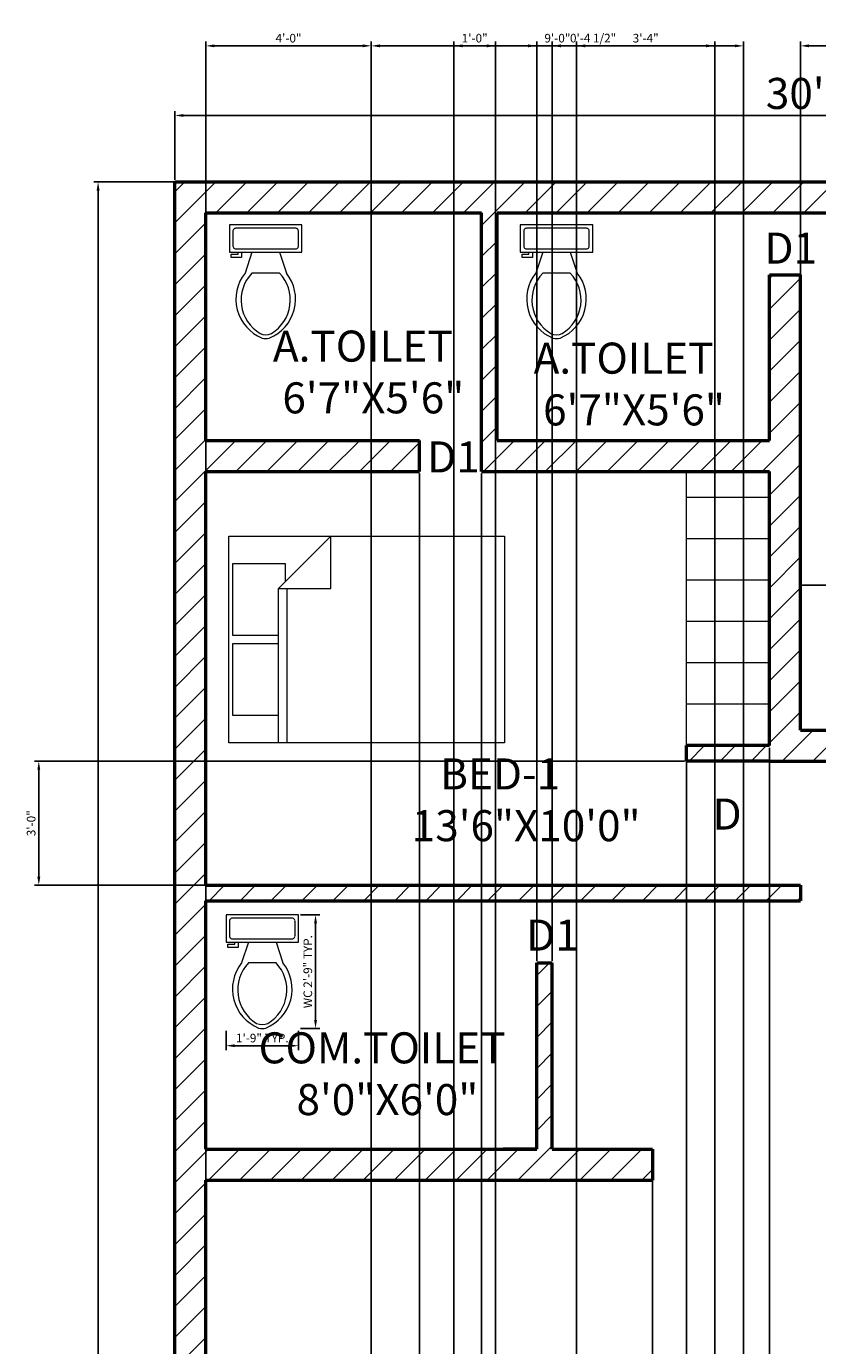
# Model space of a CAD drawing. Units: inches. Extents: x 2758 to 3288, y 1211 to 2050.
# Tile 3 of 4: x 2758 to 2988, y 1667 to 2050. Entities that reach past the tile are written whole.
import ezdxf

# ---------------------------------------------------------------- set-up
doc = ezdxf.new("R2010")
doc.units = ezdxf.units.IN
for name, color, linetype, lineweight in [('A-ANNO-DIMS', 2, 'Continuous', 18), ('A-AREA-IDEN', 7, 'Continuous', 25), ('A-FLOR-FIXT', 9, 'Continuous', 18), ('A-FURN', 8, 'Continuous', 18), ('A-WALL', 7, 'Continuous', 50)]:
    doc.layers.add(name, color=color, linetype=linetype, lineweight=lineweight)
for name, color, linetype, lineweight, true_color in [('A-ANNO-TEXT', 244, 'Continuous', 18, 0x991b1e), ('A-FLOR-CASE', 244, 'Continuous', 18, 0x991b1e), ('A-WALL-PATT', 244, 'Continuous', 13, 0x991b1e)]:
    doc.layers.add(name, color=color, linetype=linetype, lineweight=lineweight, true_color=true_color)
doc.styles.get("Standard").update_dxf_attribs({"font": 'arial.ttf'})
doc.dimstyles.new('ISO-25', dxfattribs={"dimtxt": 2.5, "dimasz": 2.5, "dimexe": 1.25, "dimexo": 0.625, "dimtad": 1, "dimlunit": 3, "dimtxsty": 'Standard', "dimcen": 2.5, "dimadec": 0, "dimazin": 0, "dimtfac": 1, "dimtmove": 0, "dimatfit": 3, "dimfxl": 1, "dimarcsym": 0})

# ---------------------------------------------------------------- blocks, each defined once
blk = doc.blocks.new('Bed - Queen')
for p, q in [((0, -80.00003), (0, 0)), ((0, 0), (59.99999, 0)), ((59.99999, 0), (59.99999, -80.00003)), ((7.99999, -1.2), (28.79998, -1.2)), ((7.99999, -14.4), (7.99999, -1.2)), ((28.79998, -1.2), (28.79998, -14.4)), ((31.19999, -1.2), (51.99999, -1.2)), ((31.19999, -14.4), (31.19999, -1.2)), ((51.99999, -1.2), (51.99999, -16.4)), ((0, -14.4), (44.8, -14.4)), ((59.99999, -29.6), (44.8, -14.4)), ((44.8, -14.4), (44.8, -29.6)), ((44.8, -16.8), (0, -16.8)), ((51.99999, -16.4), (46.79936, -16.4)), ((44.8, -29.6), (59.99999, -29.6)), ((59.99999, -80.00003), (0, -80.00003))]:
    blk.add_line(p, q)
blk = doc.blocks.new('Toilet - top')
for p, q in [((9.5, -6), (9.5, -2)), ((-10, -8.5), (-8, -8.5)), ((-10, -9.5), (-10, -8.5)), ((-7, -9.5), (-10, -9.5)), ((-8, -8.5), (-8, -8)), ((-7, -8), (-7, -9.5)), ((-4, -8), (-6, -14)), ((4, -8), (6, -14)), ((4, -14), (-4, -14))]:
    blk.add_line(p, q)
blk.add_lwpolyline([(10.5, -8), (10.5, 0), (-10.5, 0), (-10.5, -8)], close=True)
for points in [[(-9.5, -2), (-9.5, -6)], [(8.5, -1), (-8.5, -1)], [(-8.5, -7), (8.5, -7)]]:
    blk.add_lwpolyline(points)
for centre, radius, start, end in [((-8.62, -1.88), 0.884, 81.8699, 188.1301), ((8.62, -1.88), 0.884, 351.8699, 98.1301), ((-8.62, -6.12), 0.884, 171.8699, 278.1301), ((8.62, -6.12), 0.884, 261.8699, 8.1301), ((3.52, -21.58), 12.17, 141.4691, 247.9714), ((4.2, -21.82), 11.33, 136.3677, 238.9468), ((-3.52, -21.58), 12.17, 292.0284, 38.5307), ((-4.2, -21.82), 11.33, 301.053, 43.6321), ((0, -27.88), 4, 245.7318, 294.2682), ((0, -29), 4, 254.8605, 285.1395)]:
    blk.add_arc(centre, radius, start, end)
blk = doc.blocks.new('*D6')
at = {"layer": 'A-ANNO-DIMS', "color": 0, "lineweight": -2, "transparency": 16777216}
for p, q in [((2801.14, 2005.44), (2801.14, 2025.32)), ((2803.64, 2024.07), (3158.64, 2024.07)), ((3161.14, 2005.44), (3161.14, 2025.32))]:
    blk.add_line(p, q, dxfattribs=at)
at = {"layer": 'A-ANNO-DIMS', "color": 0, "transparency": 16777216}
for points in [[(2803.64, 2024.49), (2803.64, 2023.65), (2801.14, 2024.07)], [(3158.64, 2024.49), (3158.64, 2023.65), (3161.14, 2024.07)]]:
    blk.add_solid(points, dxfattribs=at)
at = {"layer": 'Defpoints', "color": 0, "transparency": 16777216}
for p in [(3161.14, 2024.07), (2801.14, 2004.81), (3161.14, 2004.81)]:
    blk.add_point(p, dxfattribs=at)
at = {"layer": 'A-ANNO-DIMS', "color": 0, "transparency": 16777216, "insert": (2981.14, 2029.29), "char_height": 9, "attachment_point": 5}
blk.add_mtext("30'", dxfattribs=at)
blk = doc.blocks.new('*D7')
at = {"layer": 'A-ANNO-DIMS', "color": 0, "lineweight": -2, "transparency": 16777216}
for p, q in [((2801.18, 2004.81), (2777.63, 2004.81)), ((2778.88, 2002.31), (2778.88, 1287.31)), ((2800.51, 1284.81), (2777.63, 1284.81))]:
    blk.add_line(p, q, dxfattribs=at)
at = {"layer": 'A-ANNO-DIMS', "color": 0, "transparency": 16777216}
for points in [[(2778.47, 2002.31), (2779.3, 2002.31), (2778.88, 2004.81)], [(2778.47, 1287.31), (2779.3, 1287.31), (2778.88, 1284.81)]]:
    blk.add_solid(points, dxfattribs=at)
at = {"layer": 'Defpoints', "color": 0, "transparency": 16777216}
for p in [(2801.81, 2004.81), (2778.88, 1284.81), (2801.14, 1284.81)]:
    blk.add_point(p, dxfattribs=at)
at = {"layer": 'A-ANNO-DIMS', "color": 0, "transparency": 16777216, "insert": (2773.66, 1644.81), "char_height": 9, "attachment_point": 5, "rotation": 90}
blk.add_mtext("60'", dxfattribs=at)
blk = doc.blocks.new('*D10')
at = {"layer": 'A-ANNO-DIMS', "color": 0, "lineweight": -2, "transparency": 16777216}
for p, q in [((2837.64, 1792.28), (2843.22, 1792.28)), ((2841.97, 1761.74), (2841.97, 1789.78)), ((2837.64, 1759.24), (2843.22, 1759.24))]:
    blk.add_line(p, q, dxfattribs=at)
at = {"layer": 'A-ANNO-DIMS', "color": 0, "transparency": 16777216}
for points in [[(2841.56, 1789.78), (2842.39, 1789.78), (2841.97, 1792.28)], [(2841.56, 1761.74), (2842.39, 1761.74), (2841.97, 1759.24)]]:
    blk.add_solid(points, dxfattribs=at)
at = {"layer": 'Defpoints', "color": 0, "transparency": 16777216}
for p in [(2837.02, 1792.28), (2841.97, 1792.28), (2837.02, 1759.24)]:
    blk.add_point(p, dxfattribs=at)
at = {"layer": 'A-ANNO-DIMS', "color": 0, "transparency": 16777216, "insert": (2840.06, 1775.76), "char_height": 2.5, "attachment_point": 5, "rotation": 90}
blk.add_mtext('WC 2\'-9" TYP.', dxfattribs=at)
blk = doc.blocks.new('*D11')
at = {"layer": 'A-ANNO-DIMS', "color": 0, "lineweight": -2, "transparency": 16777216}
for p, q in [((2816.02, 1758.61), (2816.02, 1753.03)), ((2837.02, 1758.61), (2837.02, 1753.03)), ((2818.52, 1754.28), (2834.52, 1754.28))]:
    blk.add_line(p, q, dxfattribs=at)
at = {"layer": 'A-ANNO-DIMS', "color": 0, "transparency": 16777216}
for points in [[(2818.52, 1754.7), (2818.52, 1753.86), (2816.02, 1754.28)], [(2834.52, 1754.7), (2834.52, 1753.86), (2837.02, 1754.28)]]:
    blk.add_solid(points, dxfattribs=at)
at = {"layer": 'Defpoints', "color": 0, "transparency": 16777216}
for p in [(2816.02, 1759.24), (2837.02, 1759.24), (2837.02, 1754.28)]:
    blk.add_point(p, dxfattribs=at)
at = {"layer": 'A-ANNO-DIMS', "color": 0, "transparency": 16777216, "insert": (2826.52, 1756.18), "char_height": 2.5, "attachment_point": 5}
blk.add_mtext('1\'-9" TYP.', dxfattribs=at)
blk = doc.blocks.new('*D23')
at = {"layer": 'A-ANNO-DIMS', "color": 0, "lineweight": -2, "transparency": 16777216}
for p, q in [((2903.64, 2044.26), (2901.14, 2044.26)), ((2906.14, 1778.94), (2906.14, 2045.51)), ((2906.14, 2044.26), (2910.64, 2044.26)), ((2910.64, 1778.94), (2910.64, 2045.51)), ((2913.14, 2044.26), (2929.36, 2044.26))]:
    blk.add_line(p, q, dxfattribs=at)
at = {"layer": 'A-ANNO-DIMS', "color": 0, "transparency": 16777216}
for points in [[(2903.64, 2044.68), (2903.64, 2043.84), (2906.14, 2044.26)], [(2913.14, 2044.68), (2913.14, 2043.84), (2910.64, 2044.26)]]:
    blk.add_solid(points, dxfattribs=at)
at = {"layer": 'Defpoints', "color": 0, "transparency": 16777216}
for p in [(2910.64, 2044.26), (2906.14, 1778.31), (2910.64, 1778.31)]:
    blk.add_point(p, dxfattribs=at)
at = {"layer": 'A-ANNO-DIMS', "color": 0, "transparency": 16777216, "insert": (2922.5, 2046.18), "char_height": 2.5, "attachment_point": 5}
blk.add_mtext('0\'-4 1/2"', dxfattribs=at)
blk = doc.blocks.new('*D24')
at = {"layer": 'A-ANNO-DIMS', "color": 0, "lineweight": -2, "transparency": 16777216}
for p, q in [((2872.14, 1920.19), (2872.14, 1211.4)), ((2890.14, 1920.19), (2890.14, 1211.4)), ((2874.64, 1212.65), (2887.64, 1212.65))]:
    blk.add_line(p, q, dxfattribs=at)
at = {"layer": 'A-ANNO-DIMS', "color": 0, "transparency": 16777216}
for points in [[(2874.64, 1213.06), (2874.64, 1212.23), (2872.14, 1212.65)], [(2887.64, 1213.06), (2887.64, 1212.23), (2890.14, 1212.65)]]:
    blk.add_solid(points, dxfattribs=at)
at = {"layer": 'Defpoints', "color": 0, "transparency": 16777216}
for p in [(2872.14, 1920.81), (2890.14, 1920.81), (2890.14, 1212.65)]:
    blk.add_point(p, dxfattribs=at)
at = {"layer": 'A-ANNO-DIMS', "color": 0, "transparency": 16777216, "insert": (2881.14, 1214.55), "char_height": 2.5, "attachment_point": 5}
blk.add_mtext('1\'-6"', dxfattribs=at)
blk = doc.blocks.new('*D26')
at = {"layer": 'A-ANNO-DIMS', "color": 0, "lineweight": -2, "transparency": 16777216}
for p, q in [((2949.01, 1836.81), (2760.44, 1836.81)), ((2761.69, 1803.31), (2761.69, 1834.31)), ((2982.01, 1800.81), (2760.44, 1800.81))]:
    blk.add_line(p, q, dxfattribs=at)
at = {"layer": 'A-ANNO-DIMS', "color": 0, "transparency": 16777216}
for points in [[(2761.27, 1834.31), (2762.11, 1834.31), (2761.69, 1836.81)], [(2761.27, 1803.31), (2762.11, 1803.31), (2761.69, 1800.81)]]:
    blk.add_solid(points, dxfattribs=at)
at = {"layer": 'Defpoints', "color": 0, "transparency": 16777216}
for p in [(2761.69, 1836.81), (2949.64, 1836.81), (2982.64, 1800.81)]:
    blk.add_point(p, dxfattribs=at)
at = {"layer": 'A-ANNO-DIMS', "color": 0, "transparency": 16777216, "insert": (2759.79, 1818.81), "char_height": 2.5, "attachment_point": 5, "rotation": 90}
blk.add_mtext('3\'-0"', dxfattribs=at)
blk = doc.blocks.new('*D28')
at = {"layer": 'A-ANNO-DIMS', "color": 0, "lineweight": -2, "transparency": 16777216}
for p, q in [((2939.69, 1723.69), (2939.69, 1211.4)), ((3011.14, 1723.69), (3011.14, 1211.4)), ((2942.19, 1212.65), (3008.64, 1212.65))]:
    blk.add_line(p, q, dxfattribs=at)
at = {"layer": 'A-ANNO-DIMS', "color": 0, "transparency": 16777216}
for points in [[(2942.19, 1213.06), (2942.19, 1212.23), (2939.69, 1212.65)], [(3008.64, 1213.06), (3008.64, 1212.23), (3011.14, 1212.65)]]:
    blk.add_solid(points, dxfattribs=at)
at = {"layer": 'Defpoints', "color": 0, "transparency": 16777216}
for p in [(2939.69, 1724.31), (3011.14, 1724.31), (3011.14, 1212.65)]:
    blk.add_point(p, dxfattribs=at)
at = {"layer": 'A-ANNO-DIMS', "color": 0, "transparency": 16777216, "insert": (2975.42, 1214.56), "char_height": 2.5, "attachment_point": 5}
blk.add_mtext('5\'-11 1/2"', dxfattribs=at)
blk = doc.blocks.new('*D29')
at = {"layer": 'A-ANNO-DIMS', "color": 0, "lineweight": -2, "transparency": 16777216}
for p, q in [((2858.14, 1369.44), (2858.14, 2045.51)), ((2860.64, 2044.26), (2963.64, 2044.26)), ((2966.14, 1369.44), (2966.14, 2045.51))]:
    blk.add_line(p, q, dxfattribs=at)
at = {"layer": 'A-ANNO-DIMS', "color": 0, "transparency": 16777216}
for points in [[(2860.64, 2044.68), (2860.64, 2043.84), (2858.14, 2044.26)], [(2963.64, 2044.68), (2963.64, 2043.84), (2966.14, 2044.26)]]:
    blk.add_solid(points, dxfattribs=at)
at = {"layer": 'Defpoints', "color": 0, "transparency": 16777216}
for p in [(2966.14, 2044.26), (2858.14, 1368.81), (2966.14, 1368.81)]:
    blk.add_point(p, dxfattribs=at)
at = {"layer": 'A-ANNO-DIMS', "color": 0, "transparency": 16777216, "insert": (2912.14, 2046.16), "char_height": 2.5, "attachment_point": 5}
blk.add_mtext('9\'-0"', dxfattribs=at)
blk = doc.blocks.new('*D30')
at = {"layer": 'A-ANNO-DIMS', "color": 0, "lineweight": -2, "transparency": 16777216}
for p, q in [((2882.14, 1331.94), (2882.14, 2045.51)), ((2884.64, 2044.26), (2891.64, 2044.26)), ((2894.14, 1331.94), (2894.14, 2045.51))]:
    blk.add_line(p, q, dxfattribs=at)
at = {"layer": 'A-ANNO-DIMS', "color": 0, "transparency": 16777216}
for points in [[(2884.64, 2044.68), (2884.64, 2043.84), (2882.14, 2044.26)], [(2891.64, 2044.68), (2891.64, 2043.84), (2894.14, 2044.26)]]:
    blk.add_solid(points, dxfattribs=at)
at = {"layer": 'Defpoints', "color": 0, "transparency": 16777216}
for p in [(2894.14, 2044.26), (2882.14, 1331.31), (2894.14, 1331.31)]:
    blk.add_point(p, dxfattribs=at)
at = {"layer": 'A-ANNO-DIMS', "color": 0, "transparency": 16777216, "insert": (2888.14, 2046.16), "char_height": 2.5, "attachment_point": 5}
blk.add_mtext('1\'-0"', dxfattribs=at)
blk = doc.blocks.new('*D31')
at = {"layer": 'A-ANNO-DIMS', "color": 0, "lineweight": -2, "transparency": 16777216}
for p, q in [((2810.14, 1369.44), (2810.14, 2045.51)), ((2812.64, 2044.26), (2855.64, 2044.26)), ((2858.14, 1369.44), (2858.14, 2045.51))]:
    blk.add_line(p, q, dxfattribs=at)
at = {"layer": 'A-ANNO-DIMS', "color": 0, "transparency": 16777216}
for points in [[(2812.64, 2044.68), (2812.64, 2043.84), (2810.14, 2044.26)], [(2855.64, 2044.68), (2855.64, 2043.84), (2858.14, 2044.26)]]:
    blk.add_solid(points, dxfattribs=at)
at = {"layer": 'Defpoints', "color": 0, "transparency": 16777216}
for p in [(2858.14, 2044.26), (2810.14, 1368.81), (2858.14, 1368.81)]:
    blk.add_point(p, dxfattribs=at)
at = {"layer": 'A-ANNO-DIMS', "color": 0, "transparency": 16777216, "insert": (2834.14, 2046.16), "char_height": 2.5, "attachment_point": 5}
blk.add_mtext('4\'-0"', dxfattribs=at)
blk = doc.blocks.new('*D32')
at = {"layer": 'A-ANNO-DIMS', "color": 0, "lineweight": -2, "transparency": 16777216}
for p, q in [((2949.64, 1840.69), (2949.64, 1211.4)), ((2973.64, 1840.69), (2973.64, 1211.4)), ((2952.14, 1212.65), (2971.14, 1212.65))]:
    blk.add_line(p, q, dxfattribs=at)
at = {"layer": 'A-ANNO-DIMS', "color": 0, "transparency": 16777216}
for points in [[(2952.14, 1213.06), (2952.14, 1212.23), (2949.64, 1212.65)], [(2971.14, 1213.06), (2971.14, 1212.23), (2973.64, 1212.65)]]:
    blk.add_solid(points, dxfattribs=at)
at = {"layer": 'Defpoints', "color": 0, "transparency": 16777216}
for p in [(2949.64, 1841.31), (2973.64, 1841.31), (2973.64, 1212.65)]:
    blk.add_point(p, dxfattribs=at)
at = {"layer": 'A-ANNO-DIMS', "color": 0, "transparency": 16777216, "insert": (2961.64, 1214.55), "char_height": 2.5, "attachment_point": 5}
blk.add_mtext('2\'-0"', dxfattribs=at)
blk = doc.blocks.new('*D33')
at = {"layer": 'A-ANNO-DIMS', "color": 0, "lineweight": -2, "transparency": 16777216}
for p, q in [((2983.26, 1887.81), (3023.34, 1887.81)), ((3022.09, 1885.31), (3022.09, 1848.31)), ((2983.26, 1845.81), (3023.34, 1845.81))]:
    blk.add_line(p, q, dxfattribs=at)
at = {"layer": 'A-ANNO-DIMS', "color": 0, "transparency": 16777216}
for points in [[(3021.67, 1885.31), (3022.51, 1885.31), (3022.09, 1887.81)], [(3021.67, 1848.31), (3022.51, 1848.31), (3022.09, 1845.81)]]:
    blk.add_solid(points, dxfattribs=at)
at = {"layer": 'Defpoints', "color": 0, "transparency": 16777216}
for p in [(2982.64, 1887.81), (2982.64, 1845.81), (3022.09, 1845.81)]:
    blk.add_point(p, dxfattribs=at)
at = {"layer": 'A-ANNO-DIMS', "color": 0, "transparency": 16777216, "insert": (3020.19, 1866.81), "char_height": 2.5, "attachment_point": 5, "rotation": 90}
blk.add_mtext('3\'-6"', dxfattribs=at)
blk = doc.blocks.new('*D34')
at = {"layer": 'A-ANNO-DIMS', "color": 0, "lineweight": -2, "transparency": 16777216}
for p, q in [((2982.64, 1888.44), (2982.64, 2045.51)), ((2985.14, 2044.26), (3107.64, 2044.26)), ((3110.14, 1888.44), (3110.14, 2045.51))]:
    blk.add_line(p, q, dxfattribs=at)
at = {"layer": 'A-ANNO-DIMS', "color": 0, "transparency": 16777216}
for points in [[(2985.14, 2044.68), (2985.14, 2043.84), (2982.64, 2044.26)], [(3107.64, 2044.68), (3107.64, 2043.84), (3110.14, 2044.26)]]:
    blk.add_solid(points, dxfattribs=at)
at = {"layer": 'Defpoints', "color": 0, "transparency": 16777216}
for p in [(3110.14, 2044.26), (2982.64, 1887.81), (3110.14, 1887.81)]:
    blk.add_point(p, dxfattribs=at)
at = {"layer": 'A-ANNO-DIMS', "color": 0, "transparency": 16777216, "insert": (3046.39, 2046.18), "char_height": 2.5, "attachment_point": 5}
blk.add_mtext('10\'-7 1/2"', dxfattribs=at)
blk = doc.blocks.new('*D35')
at = {"layer": 'A-ANNO-DIMS', "color": 0, "lineweight": -2, "transparency": 16777216}
for p, q in [((2917.71, 1560.11), (2917.71, 2045.51)), ((2920.21, 2044.26), (2955.28, 2044.26)), ((2957.78, 1560.11), (2957.78, 2045.51))]:
    blk.add_line(p, q, dxfattribs=at)
at = {"layer": 'A-ANNO-DIMS', "color": 0, "transparency": 16777216}
for points in [[(2920.21, 2044.68), (2920.21, 2043.84), (2917.71, 2044.26)], [(2955.28, 2044.68), (2955.28, 2043.84), (2957.78, 2044.26)]]:
    blk.add_solid(points, dxfattribs=at)
at = {"layer": 'Defpoints', "color": 0, "transparency": 16777216}
for p in [(2957.78, 2044.26), (2917.71, 1559.49), (2957.78, 1559.49)]:
    blk.add_point(p, dxfattribs=at)
at = {"layer": 'A-ANNO-DIMS', "color": 0, "transparency": 16777216, "insert": (2937.75, 2046.16), "char_height": 2.5, "attachment_point": 5}
blk.add_mtext('3\'-4"', dxfattribs=at)

msp = doc.modelspace()

# ---------------------------------------------------------------- hatches: boundary and pattern name
at = {"layer": 'A-WALL-PATT'}
h = msp.add_hatch(dxfattribs=at)
h.set_pattern_fill('ANSI31', color=256, scale=2)
h.paths.add_polyline_path([(2810.139, 1377.81), (2810.139, 1715.31), (2939.691, 1715.31), (2939.691, 1724.31), (2910.639, 1724.31), (2910.639, 1778.31), (2906.139, 1778.31), (2906.139, 1724.31), (2896.389, 1724.31), (2810.139, 1724.31), (2810.139, 1796.31), (2982.639, 1796.31), (2982.639, 1800.81), (2810.139, 1800.81), (2810.139, 1920.81), (2872.139, 1920.81), (2872.139, 1929.81), (2810.139, 1929.81), (2810.139, 1995.81), (2890.139, 1995.81), (2890.139, 1920.81), (2973.639, 1920.81), (2973.639, 1841.31), (2949.639, 1841.31), (2949.639, 1836.81), (2973.639, 1836.81), (3114.639, 1836.81), (3114.639, 1887.81), (3110.139, 1887.81), (3110.139, 1845.81), (2982.639, 1845.81), (2982.639, 1977.81), (2973.639, 1977.81), (2973.639, 1929.81), (2894.639, 1929.81), (2894.639, 1995.81), (3152.139, 1995.81), (3152.139, 1800.81), (3152.139, 1796.31), (3152.139, 1724.31), (3074.139, 1724.31), (3074.139, 1715.31), (3152.139, 1715.31), (3152.139, 1595.31), (3020.139, 1595.31), (3020.139, 1667.31), (3011.139, 1667.31), (3011.139, 1586.31), (3080.139, 1586.31), (3080.139, 1284.81), (3089.139, 1284.81), (3089.139, 1586.31), (3161.139, 1586.31), (3161.139, 2004.81), (2801.139, 2004.81), (2801.139, 1284.81), (3032.139, 1284.81), (3032.139, 1320.81), (3023.139, 1320.81), (3023.139, 1293.81), (2810.139, 1293.81), (2810.139, 1368.81), (3032.139, 1368.81), (3032.139, 1377.81)])

# ---------------------------------------------------------------- linework, layer by layer
at = {"layer": 'A-FLOR-CASE'}
for p, q in [((2949.639, 1836.81), (2949.639, 1920.81)), ((2973.639, 1913.31), (2949.639, 1913.31)), ((2973.639, 1901.31), (2949.639, 1901.31)), ((2973.639, 1889.31), (2949.639, 1889.31)), ((2982.639, 1887.81), (3114.639, 1887.81)), ((2973.639, 1877.31), (2949.639, 1877.31)), ((2973.639, 1865.31), (2949.639, 1865.31)), ((2973.639, 1853.31), (2949.639, 1853.31))]:
    msp.add_line(p, q, dxfattribs=at)
at = {"layer": 'A-WALL'}
for p, q in [((2801.139, 2004.81), (3161.139, 2004.81)), ((2801.139, 1284.81), (2801.139, 2004.81)), ((2810.139, 1995.81), (2890.139, 1995.81)), ((2810.139, 1929.81), (2810.139, 1995.81)), ((2890.139, 1920.81), (2890.139, 1995.81)), ((2894.639, 1929.81), (2894.639, 1995.81)), ((2894.639, 1995.81), (3152.139, 1995.81)), ((2973.639, 1977.81), (2982.639, 1977.81)), ((2973.639, 1929.81), (2973.639, 1977.81)), ((2982.639, 1845.81), (2982.639, 1977.81)), ((2810.139, 1929.81), (2872.139, 1929.81)), ((2872.139, 1920.81), (2872.139, 1929.81)), ((2894.639, 1929.81), (2973.639, 1929.81)), ((2810.139, 1920.81), (2872.139, 1920.81)), ((2810.139, 1800.81), (2810.139, 1920.81)), ((2890.139, 1920.81), (2973.639, 1920.81)), ((2973.639, 1841.31), (2973.639, 1920.81)), ((2982.639, 1845.81), (2982.639, 1920.81)), ((2982.639, 1845.81), (3110.139, 1845.81)), ((2949.639, 1836.81), (2949.639, 1841.31)), ((2973.639, 1841.31), (2949.639, 1841.31)), ((2973.639, 1836.81), (2949.639, 1836.81)), ((2973.639, 1836.81), (3114.639, 1836.81)), ((2810.139, 1800.81), (2982.639, 1800.81)), ((2982.639, 1800.81), (2982.639, 1796.31)), ((2810.139, 1796.31), (2982.639, 1796.31)), ((2810.139, 1724.31), (2810.139, 1796.31)), ((2906.139, 1724.31), (2906.139, 1778.31)), ((2906.139, 1778.31), (2910.639, 1778.31)), ((2910.639, 1724.31), (2910.639, 1778.31)), ((2810.139, 1724.31), (2906.139, 1724.31)), ((2906.139, 1724.31), (2896.389, 1724.31)), ((2910.639, 1724.31), (2939.691, 1724.31)), ((2939.691, 1724.31), (2939.691, 1715.31)), ((2810.139, 1715.31), (2939.691, 1715.31)), ((2810.139, 1523.31), (2810.139, 1715.31))]:
    msp.add_line(p, q, dxfattribs=at)

# ---------------------------------------------------------------- block references
at = {"layer": 'A-FLOR-FIXT'}
for p in [(2827.519, 1992.379), (2911.877, 1992.379), (2826.517, 1792.283)]:
    msp.add_blockref('Toilet - top', p, dxfattribs=at)
at = {"layer": 'A-FURN', "rotation": 90}
msp.add_blockref('Bed - Queen', (2816.802, 1842.099), dxfattribs=at)

# ---------------------------------------------------------------- texts
at = {"layer": 'A-ANNO-TEXT', "char_height": 9, "attachment_point": 1}
for s, width, heights, insert in [('D1', 12.06443, [0], (2972.205, 1990.089)), ('D1', 12.06443, [0], (2874.363, 1929.546)), ('D', 20.63641, [11.065], (2957.146, 1825.967)), ('D1', 12.06443, [0], (2903.093, 1790.86))]:
    msp.add_mtext_dynamic_manual_height_columns(s, width=width, gutter_width=12.5, heights=heights, dxfattribs=dict(at, insert=insert))
at = {"layer": 'A-AREA-IDEN', "char_height": 9, "attachment_point": 1}
for s, insert in [(' A.TOILET\\P  6\'7"X5\'6"', (2826.859, 1961.678)), (' A.TOILET\\P  6\'7"X5\'6"', (2902.489, 1958.19)), ('   BED-1\\P13\'6"X10\'0"', (2869.885, 1837.602)), (' COM.TOILET\\P     8\'0"X6\'0"', (2822.702, 1758.162))]:
    msp.add_mtext_dynamic_manual_height_columns(s, width=130.32194, gutter_width=12.5, heights=[77.844], dxfattribs=dict(at, insert=insert))

# ---------------------------------------------------------------- dimensions: what is measured, and where the dimension line sits
at = {"layer": 'A-ANNO-DIMS'}
for base, p1, p2, override, picture, middle in [((2858.139, 2044.26), (2810.139, 1368.81), (2858.139, 1368.81), {"dimdec": 1, "dimlfac": 1, "dimrnd": 0, "dimzin": 1, "dimdsep": 46, "dimlunit": 4, "dimfrac": 2}, '*D31', (2834.139, 2046.162)), ((2966.139, 2044.26), (2858.139, 1368.81), (2966.139, 1368.81), {"dimdec": 1, "dimlfac": 1, "dimrnd": 0, "dimzin": 1, "dimdsep": 46, "dimlunit": 4, "dimfrac": 2}, '*D29', (2912.139, 2046.162)), ((2894.139, 2044.26), (2882.139, 1331.31), (2894.139, 1331.31), {"dimdec": 1, "dimlfac": 1, "dimrnd": 0, "dimzin": 1, "dimdsep": 46, "dimlunit": 4, "dimfrac": 2}, '*D30', (2888.139, 2046.162)), ((2910.639, 2044.26), (2906.139, 1778.31), (2910.639, 1778.31), {"dimdec": 1, "dimlfac": 1, "dimrnd": 0, "dimzin": 1, "dimdsep": 46, "dimlunit": 4, "dimfrac": 2}, '*D23', (2922.499, 2046.178)), ((2957.785, 2044.26), (2917.71, 1559.489), (2957.785, 1559.489), {"dimdec": 1, "dimlfac": 1, "dimrnd": 0, "dimzin": 1, "dimdsep": 46, "dimlunit": 4, "dimfrac": 2}, '*D35', (2937.747, 2046.163)), ((3110.139, 2044.26), (2982.639, 1887.81), (3110.139, 1887.81), {"dimdec": 1, "dimlfac": 1, "dimrnd": 0, "dimzin": 1, "dimdsep": 46, "dimlunit": 4, "dimfrac": 2}, '*D34', (3046.389, 2046.178)), ((3161.139, 2024.068), (2801.139, 2004.81), (3161.139, 2004.81), {"dimtxt": 9, "dimclrd": 0, "dimclre": 0, "dimclrt": 0}, '*D6', (2981.139, 2029.292)), ((2890.139, 1212.647), (2872.139, 1920.81), (2890.139, 1920.81), {"dimdec": 1, "dimlfac": 1, "dimrnd": 0, "dimzin": 1, "dimdsep": 46, "dimlunit": 4, "dimfrac": 2}, '*D24', (2881.139, 1214.549)), ((2973.639, 1212.647), (2949.639, 1841.31), (2973.639, 1841.31), {"dimdec": 1, "dimlfac": 1, "dimrnd": 0, "dimzin": 1, "dimdsep": 46, "dimlunit": 4, "dimfrac": 2}, '*D32', (2961.639, 1214.549)), ((3011.139, 1212.647), (2939.691, 1724.31), (3011.139, 1724.31), {"dimdec": 1, "dimlfac": 1, "dimrnd": 0, "dimzin": 1, "dimdsep": 46, "dimlunit": 4, "dimfrac": 2}, '*D28', (2975.415, 1214.565))]:
    dim = msp.add_linear_dim(base=base, p1=p1, p2=p2, dimstyle='ISO-25', override=override, dxfattribs=at)
    dim.commit()
    dim.dimension.update_dxf_attribs({"geometry": picture, "text_midpoint": middle})
for base, p1, p2, angle, override, picture, middle in [((2778.882, 1284.81), (2801.807, 2004.81), (2801.139, 1284.81), 90, {"dimtxt": 9, "dimclrd": 0, "dimclre": 0, "dimclrt": 0}, '*D7', (2773.662, 1644.81)), ((3022.089, 1845.81), (2982.639, 1887.81), (2982.639, 1845.81), 270, {"dimdec": 1, "dimlfac": 1, "dimrnd": 0, "dimzin": 1, "dimdsep": 46, "dimlunit": 4, "dimfrac": 2}, '*D33', (3020.187, 1866.81)), ((2761.689, 1836.81), (2982.639, 1800.81), (2949.639, 1836.81), 90, {"dimdec": 1, "dimlfac": 1, "dimrnd": 0, "dimzin": 1, "dimdsep": 46, "dimlunit": 4, "dimfrac": 2}, '*D26', (2759.787, 1818.81))]:
    dim = msp.add_linear_dim(base=base, p1=p1, p2=p2, angle=angle, dimstyle='ISO-25', override=override, dxfattribs=at)
    dim.commit()
    dim.dimension.update_dxf_attribs({"geometry": picture, "text_midpoint": middle})
dim = msp.add_linear_dim(base=(2841.974, 1792.283), p1=(2837.017, 1759.237), p2=(2837.017, 1792.283), angle=90, text='WC <> TYP.', dimstyle='ISO-25', override={"dimdec": 1, "dimlfac": 1, "dimrnd": 0, "dimzin": 1, "dimdsep": 46, "dimlunit": 4, "dimfrac": 2}, dxfattribs=at)
dim.commit()
dim.dimension.update_dxf_attribs({"geometry": '*D10', "text_midpoint": (2840.056, 1775.76)})
dim = msp.add_linear_dim(base=(2837.017, 1754.28), p1=(2816.017, 1759.237), p2=(2837.017, 1759.237), text='<> TYP.', dimstyle='ISO-25', override={"dimdec": 1, "dimlfac": 1, "dimrnd": 0, "dimzin": 1, "dimdsep": 46, "dimlunit": 4, "dimfrac": 2}, dxfattribs=at)
dim.commit()
dim.dimension.update_dxf_attribs({"geometry": '*D11', "text_midpoint": (2826.517, 1756.181)})

doc.saveas('drawing.dxf')
